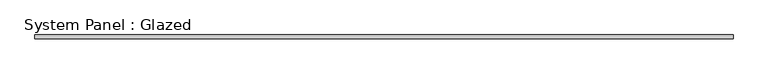
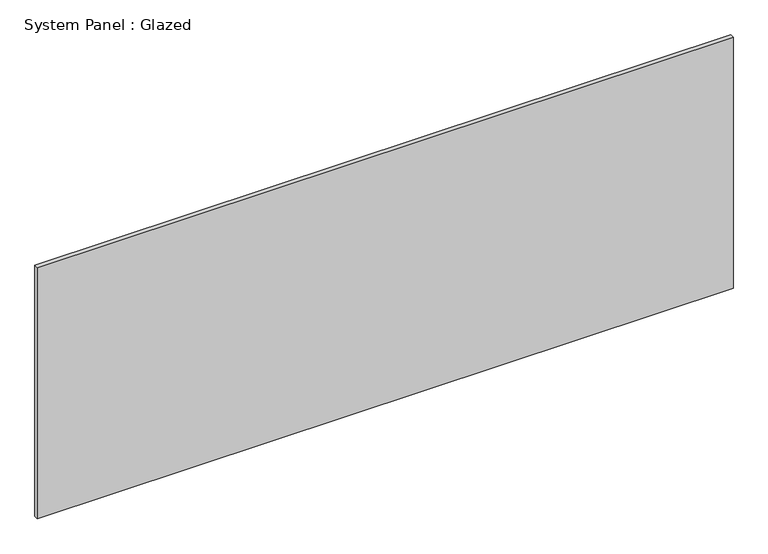
"""IFC4 building model written with IfcOpenShell, lengths in millimetres: plate geometry, System Panel : Glazed."""

from ifc_helpers import new_model, si_unit, origin, origin_with_axes, place, context, project, spatial, polyline, outline, extrude, source, transform, mapped, element, save


def system_panel_glazed_ed669c81(model_context):
    return source(origin(), model_context, "Body", "SweptSolid", [
        extrude(outline(polyline([(2314.575, 19.05), (-2314.575, 19.05), (-2314.575, 44.45), (2314.575, 44.45), (2314.575, 19.05)])), origin_with_axes(), (0.0, 0.0, 1.0), 1765.3),
    ])


if __name__ == "__main__":
    model = new_model("IFC4")
    model_context = context("Model", 3, world=origin())
    ifc_project = project(units=[si_unit("LENGTHUNIT", "METRE", prefix="MILLI")], contexts=[model_context])
    site = spatial("IfcSite", under=ifc_project)
    building = spatial("IfcBuilding", under=site)
    placement = place(None, origin())
    system_panel_glazed_shape = system_panel_glazed_ed669c81(model_context)
    element("IfcPlate", 1, ObjectType="System Panel : Glazed", at=placement, inside=building, context=model_context, shape_type="MappedRepresentation", body=[
        mapped(system_panel_glazed_shape, transform((0.0, 0.0, 0.0), x_axis=(1.0, 0.0, 0.0), y_axis=(0.0, 1.0, 0.0), z_axis=(0.0, 0.0, 1.0))),
    ])
    save(model, "model.ifc")

# Revit data of these elements
# Type "System Panel : Glazed"
#   Construction Type Id = "GSP4R"
#   Analytic Construction = "1/8 in Pilkington single glazing"
#   Visual Light Transmittance = 0.9
#   Solar Heat Gain Coefficient = 0.86
#   Heat Transfer Coefficient (U) = 1.18115 BTU/(h·ft²·°F)
# Element 1 (IfcPlate, "System Panel : Glazed")
#   Materials on its faces: "Glass"
# Materials
#   "Glass": class "Glass", colour RGB 0 128 192, transparency 0.75, Description = "Soda Lime Glass", Cost = 0
